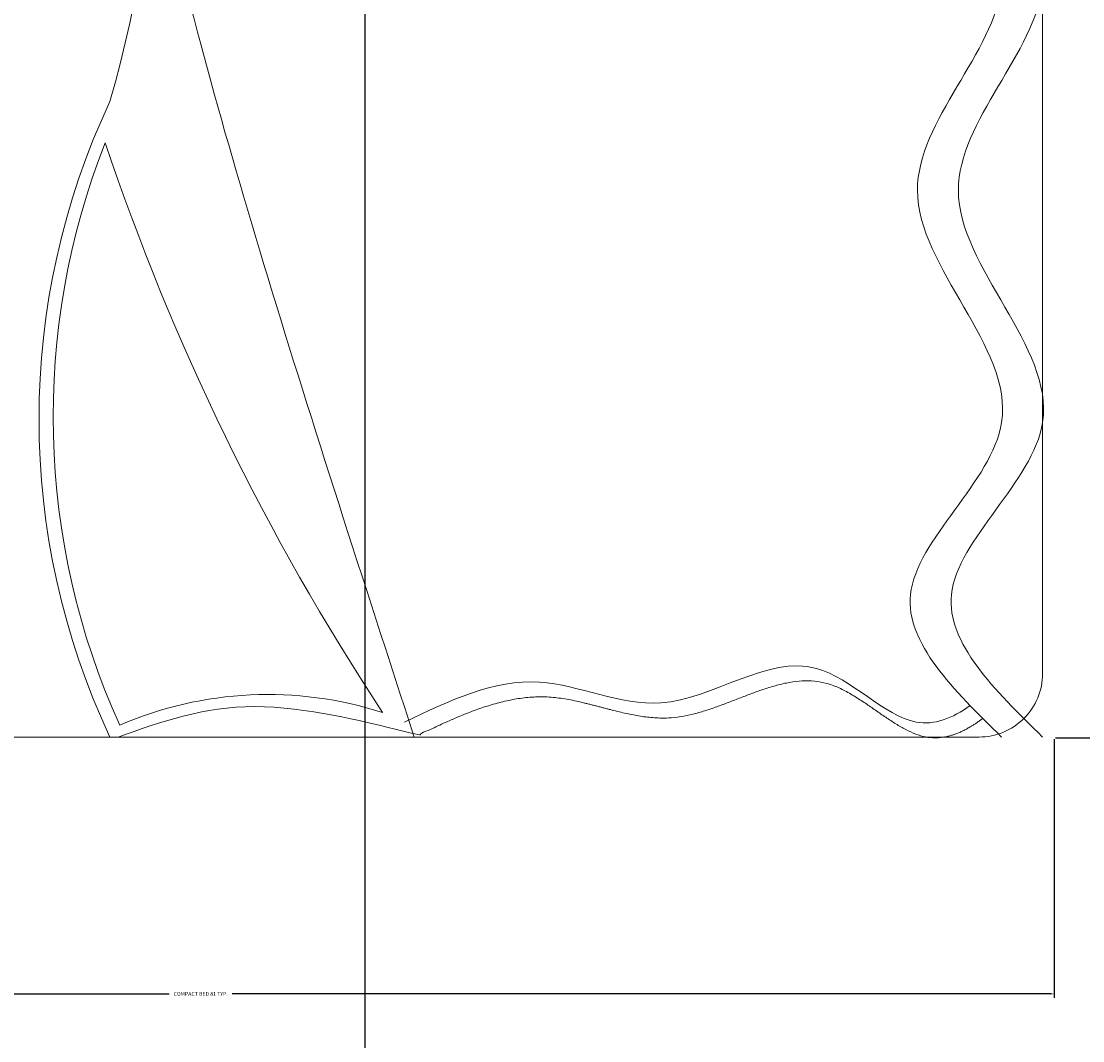
# Model space of a CAD drawing. Units: inches. Extents: x -61 to 1599, y -1316 to 257.
# Tile 148 of 204: x 440 to 490, y 52 to 101. Entities that reach past the tile are written whole.
import ezdxf

# ---------------------------------------------------------------- set-up
doc = ezdxf.new("R2010")
doc.units = ezdxf.units.IN
doc.header["$MEASUREMENT"] = 0
doc.layers.add('A-ANNO-DIMS', color=2, linetype='Continuous', lineweight=18)
doc.layers.add('FURNITURE', color=83, linetype='Continuous', lineweight=18)
doc.styles.get("Standard").update_dxf_attribs({"font": 'arial.ttf'})
doc.dimstyles.get("Standard").update_dxf_attribs({"dimtxt": 0.18, "dimasz": 0.18, "dimexe": 0.18, "dimexo": 0.0625, "dimgap": 0.09, "dimtad": 0, "dimtih": 1, "dimtoh": 1, "dimdec": 0, "dimzin": 0, "dimdsep": 46, "dimlunit": 3, "dimtxsty": 'Standard', "dimcen": 0.09, "dimadec": 0, "dimazin": 0, "dimtfac": 1, "dimtdec": 0, "dimtofl": 0, "dimtmove": 0, "dimatfit": 3, "dimfxl": 1, "dimtolj": 1, "dimtzin": 0, "dimarcsym": 0})

# ---------------------------------------------------------------- blocks, each defined once
blk = doc.blocks.new('BED-DOUBLE-COMPACT')
for points in [[(77, 60.036), (3, 60.036, 0.414214), (0, 57.036), (0, 3.036, 0.414214), (3, 0.036), (77, 0.036, 0.414214), (80, 3.036), (80, 57.036, 0.414214)], [(35.767, 28.086, 0.064396), (48.861, 1.193, 0.181766), (36.455, 0.601, -0.202767)]]:
    blk.add_lwpolyline(points, format="xyb", close=True)
blk.add_lwpolyline([(35.995, 0.036, -0.22309), (35.995, 30.036, 0.142156), (35.995, 60.036)], format="xyb")
for points, weights, knots in [([(50.356, 0.036), (44.305, 9.081), (39.572, 18.88), (36.247, 29.242), (36.329, 29.431), (36.413, 29.619), (36.498, 29.807), (39.384, 39.751), (39.361, 50.105), (36.431, 60.036), (39.05, 58.775), (44.504, 56.147), (52.793, 61.024), (60.854, 55.204), (67.651, 61.048), (73.388, 57.356), (75.556, 56.449)], [1, 0.993520320424, 0.993520320424, 1, 0.99997444972, 0.99997444972, 1, 0.973174868659, 0.973174868659, 1, 1, 1, 1, 1, 1, 1, 1], [0, 0, 0, 0, 0.279074, 0.279074, 0.279074, 0.296584, 0.296584, 0.296584, 0.865868, 0.865868, 0.865868, 9.142578, 18.107734, 25.769226, 34.110801, 40.441511, 40.441511, 40.441511, 40.441511]), ([(36.376, 0.036), (40.901, 1.989), (45.83, 1.989), (50.356, 0.036), (52.467, 1.047), (56.421, 2.94), (63.004, -0.478), (69.272, 4.675), (73.916, -0.767), (76.296, 0.253), (77.177, 0.915)], [1, 0.945466318698, 0.945466318698, 1, 1, 1, 1, 1, 1, 1, 1], [0, 0, 0, 0, 0.814571, 0.814571, 0.814571, 7.464247, 13.266353, 20.788537, 26.138745, 29.321895, 29.321895, 29.321895, 29.321895])]:
    blk.add_rational_spline(points, weights, degree=3, knots=knots)
for points, knots in [([(78.068, 0.036), (75.8, 2.259), (70.917, 7.043), (82.188, 15.495), (70.028, 25.556), (82.2, 36.262), (68.972, 47.493), (74.957, 55.746), (78.068, 60.036)], [0, 0, 0, 0, 7.980285, 17.179806, 28.830278, 39.318084, 52.078264, 65.891546, 65.891546, 65.891546, 65.891546]), ([(80, 0.036), (77.732, 2.259), (72.849, 7.043), (84.121, 15.495), (71.96, 25.556), (84.132, 36.262), (70.904, 47.493), (76.889, 55.746), (80, 60.036)], [0, 0, 0, 0, 7.980285, 17.179806, 28.830278, 39.318084, 52.078264, 65.891546, 65.891546, 65.891546, 65.891546]), ([(49.888, 0.742), (51.999, 1.752), (55.953, 3.645), (62.536, 0.227), (68.803, 5.38), (73.403, -0.008), (75.74, 0.922), (76.578, 1.524)], [0, 0, 0, 0, 6.649676, 12.451782, 19.973966, 25.324174, 28.349676, 28.349676, 28.349676, 28.349676])]:
    blk.add_open_spline(points, degree=3, knots=knots)
blk = doc.blocks.new('*D676')
at = {"layer": 'A-ANNO-DIMS', "color": 0, "lineweight": -2, "transparency": 16777216}
for p, q in [((407.794, 66.667), (407.794, 54.467)), ((488.345, 66.667), (488.345, 54.467)), ((407.974, 54.647), (446.586, 54.647)), ((488.165, 54.647), (449.554, 54.647))]:
    blk.add_line(p, q, dxfattribs=at)
at = {"layer": 'A-ANNO-DIMS', "color": 0, "transparency": 16777216}
for points in [[(407.974, 54.677), (407.974, 54.617), (407.794, 54.647)], [(488.165, 54.677), (488.165, 54.617), (488.345, 54.647)]]:
    blk.add_solid(points, dxfattribs=at)
at = {"layer": 'DEFPOINTS', "color": 0, "transparency": 16777216}
for p in [(407.794, 66.729), (488.345, 66.729), (488.345, 54.647)]:
    blk.add_point(p, dxfattribs=at)
at = {"layer": 'A-ANNO-DIMS', "color": 0, "transparency": 16777216, "insert": (448.07, 54.647), "char_height": 0.18, "attachment_point": 5}
blk.add_mtext('\\A1;COMPACT BED 81 TYP.', dxfattribs=at)
blk = doc.blocks.new('*D677')
at = {"layer": 'A-ANNO-DIMS', "color": 0, "lineweight": -2, "transparency": 16777216}
for p, q in [((488.407, 129.084), (500.607, 129.084)), ((500.427, 128.904), (500.427, 98.089)), ((500.427, 66.909), (500.427, 97.725)), ((488.407, 66.729), (500.607, 66.729))]:
    blk.add_line(p, q, dxfattribs=at)
at = {"layer": 'A-ANNO-DIMS', "color": 0, "transparency": 16777216}
for points in [[(500.397, 128.904), (500.457, 128.904), (500.427, 129.084)], [(500.397, 66.909), (500.457, 66.909), (500.427, 66.729)]]:
    blk.add_solid(points, dxfattribs=at)
at = {"layer": 'DEFPOINTS', "color": 0, "transparency": 16777216}
for p in [(488.345, 129.084), (500.427, 129.084), (488.345, 66.729)]:
    blk.add_point(p, dxfattribs=at)
at = {"layer": 'A-ANNO-DIMS', "color": 0, "transparency": 16777216, "insert": (500.427, 97.907), "char_height": 0.18, "attachment_point": 5}
blk.add_mtext('\\A1;62 TYP.', dxfattribs=at)
blk = doc.blocks.new('*D703')
at = {"layer": 'A-ANNO-DIMS', "color": 0, "lineweight": -2, "transparency": 16777216}
for p, q in [((372.32, -616.882), (372.32, 257.457)), ((455.833, -616.882), (455.833, 257.457)), ((372.5, 257.277), (413.7, 257.277)), ((455.653, 257.277), (414.453, 257.277))]:
    blk.add_line(p, q, dxfattribs=at)
at = {"layer": 'A-ANNO-DIMS', "color": 0, "transparency": 16777216}
for points in [[(372.5, 257.307), (372.5, 257.247), (372.32, 257.277)], [(455.653, 257.307), (455.653, 257.247), (455.833, 257.277)]]:
    blk.add_solid(points, dxfattribs=at)
at = {"layer": 'DEFPOINTS', "color": 0, "transparency": 16777216}
for p in [(455.833, 257.277), (372.32, -616.945), (455.833, -616.945)]:
    blk.add_point(p, dxfattribs=at)
at = {"layer": 'A-ANNO-DIMS', "color": 0, "transparency": 16777216, "insert": (414.076, 257.277), "char_height": 0.18, "attachment_point": 5}
blk.add_mtext('\\A1;83.51', dxfattribs=at)

msp = doc.modelspace()

# ---------------------------------------------------------------- block references
at = {"layer": 'FURNITURE'}
msp.add_blockref('BED-DOUBLE-COMPACT', (407.794, 66.733), dxfattribs=at)

# ---------------------------------------------------------------- dimensions: what is measured, and where the dimension line sits
at = {"layer": 'A-ANNO-DIMS'}
dim = msp.add_linear_dim(base=(455.8327, 257.2771), p1=(372.3201, -616.9446), p2=(455.8327, -616.9446), dimstyle='Standard', override={"dimdec": 2, "dimlfac": 1, "dimrnd": 0, "dimzin": 0, "dimdsep": 46, "dimlunit": 2}, dxfattribs=at)
dim.commit()
dim.dimension.update_dxf_attribs({"geometry": '*D703', "text_midpoint": (414.0764, 257.2771)})
dim = msp.add_linear_dim(base=(500.4274, 129.084), p1=(488.3448, 66.7295), p2=(488.3448, 129.084), angle=90, text='<> TYP.', dimstyle='Standard', override={"dimdec": 0, "dimlfac": 1, "dimrnd": 0, "dimzin": 0, "dimdsep": 46, "dimlunit": 2}, dxfattribs=at)
dim.commit()
dim.dimension.update_dxf_attribs({"geometry": '*D677', "text_midpoint": (500.4274, 97.9068)})
dim = msp.add_linear_dim(base=(488.3448, 54.6469), p1=(407.7945, 66.7295), p2=(488.3448, 66.7295), text='COMPACT BED <> TYP.', dimstyle='Standard', override={"dimdec": 0, "dimlfac": 1, "dimrnd": 0, "dimzin": 0, "dimdsep": 46, "dimlunit": 2}, dxfattribs=at)
dim.commit()
dim.dimension.update_dxf_attribs({"geometry": '*D676', "text_midpoint": (448.0696, 54.6469)})

doc.saveas('drawing.dxf')
